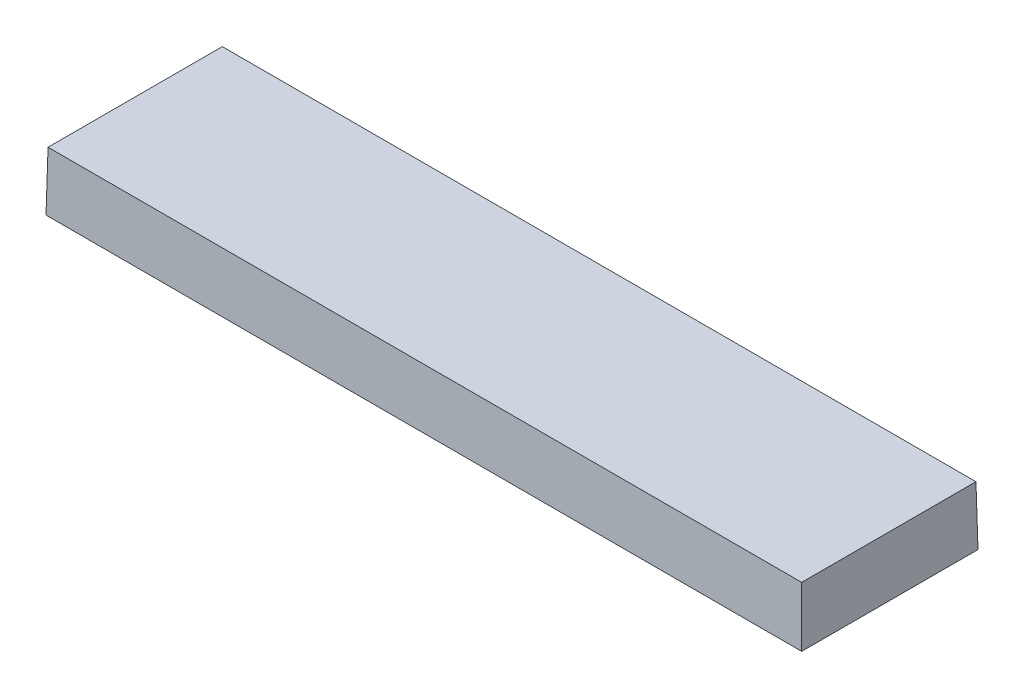
from build123d import *

# Parameters (mm, degrees)
COTTER_PROFILE_90X25_W          = 90
COTTER_PROFILE_90X25_H          = 21
COTTER_BODY_7MM_DRAFTED_1_DEPTH = 7
COTTER_BODY_7MM_DRAFTED_1_TAPER = 1


with BuildPart() as part:
    # Cotter Profile 90x25 → Cotter Body 7mm Drafted 1° (new body)
    with BuildSketch(Plane(origin=(0, 0, 0), x_dir=(1, 0, 0), z_dir=(0, 1, 0))):
        Rectangle(COTTER_PROFILE_90X25_W, COTTER_PROFILE_90X25_H)
    extrude(amount=COTTER_BODY_7MM_DRAFTED_1_DEPTH, taper=COTTER_BODY_7MM_DRAFTED_1_TAPER)


solid = part.part
